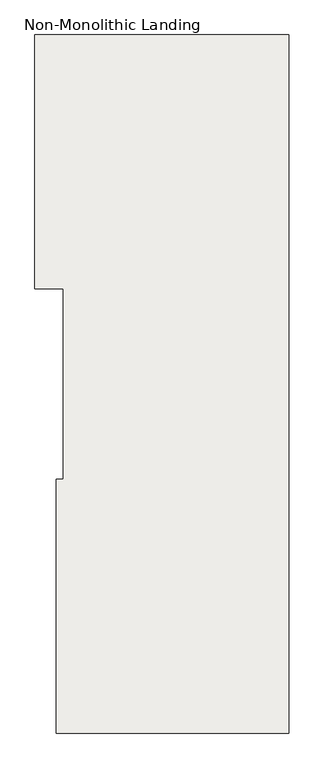
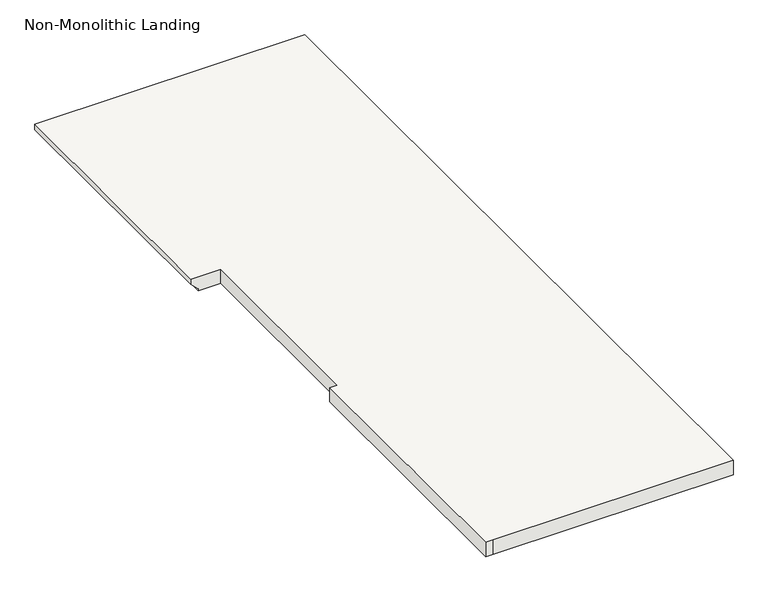
"""IFC4 building model written with IfcOpenShell, lengths in millimetres: slab geometry, Non-Monolithic Landing."""

from ifc_helpers import new_model, si_unit, origin, place, context, project, spatial, faceted_brep, source, transform, mapped, element, save


def non_monolithic_landing_c967b2c0(model_context):
    return source(origin(), model_context, "Body", "Brep", [
        faceted_brep([(-4002.2725091, 10512.3149226, 1674.2833333), (-4002.2725091, 10512.3149226, 1693.3333333), (-4002.2725091, 11426.7149226, 1693.3333333), (-4002.2725091, 11426.7149226, 1674.2833333), (-3976.8725091, 10512.3149226, 1648.8833333), (-3976.8725091, 11426.7149226, 1648.8833333), (-3900.6725091, 10512.3149226, 1693.3333333), (-3900.6725091, 9826.5149226, 1693.3333333), (-3926.0725091, 9826.5149226, 1693.3333333), (-3926.0725091, 8912.1149226, 1693.3333333), (-3900.6725091, 8912.1149226, 1693.3333333), (-3087.8725091, 8912.1149226, 1693.3333333), (-3087.8725091, 11426.7149226, 1693.3333333), (-3976.8725091, 10512.3149226, 1642.5333333), (-3976.8725091, 11426.7149226, 1642.5333333), (-3087.8725091, 11426.7149226, 1642.5333333), (-3087.8725091, 8912.1149226, 1642.5333333), (-3900.6725091, 8912.1149226, 1642.5333333), (-3926.0725091, 8912.1149226, 1642.5333333), (-3926.0725091, 9826.5149226, 1642.5333333), (-3900.6725091, 9826.5149226, 1642.5333333), (-3900.6725091, 10512.3149226, 1642.5333333)], [[[0, 1, 2, 3]], [[4, 0, 3, 5]], [[6, 7, 8, 9, 10, 11, 12, 2, 1]], [[13, 14, 15, 16, 17, 18, 19, 20, 21]], [[14, 13, 4, 5]], [[6, 1, 0, 4, 13, 21]], [[11, 10, 17, 16]], [[12, 11, 16, 15]], [[2, 12, 15, 14, 5, 3]], [[7, 6, 21, 20]], [[8, 7, 20, 19]], [[9, 8, 19, 18]], [[10, 9, 18, 17]]]),
    ])


if __name__ == "__main__":
    model = new_model("IFC4")
    model_context = context("Model", 3, world=origin())
    ifc_project = project(units=[si_unit("LENGTHUNIT", "METRE", prefix="MILLI")], contexts=[model_context])
    site = spatial("IfcSite", under=ifc_project)
    building = spatial("IfcBuilding", under=site)
    placement = place(None, origin())
    non_monolithic_landing_shape = non_monolithic_landing_c967b2c0(model_context)
    element("IfcSlab", 1, ObjectType="Non-Monolithic Landing", at=placement, inside=building, context=model_context, shape_type="MappedRepresentation", body=[
        mapped(non_monolithic_landing_shape, transform((0.0, 0.0, 0.0), x_axis=(1.0, 0.0, 0.0), y_axis=(0.0, 1.0, 0.0), z_axis=(0.0, 0.0, 1.0))),
    ])
    save(model, "model.ifc")
